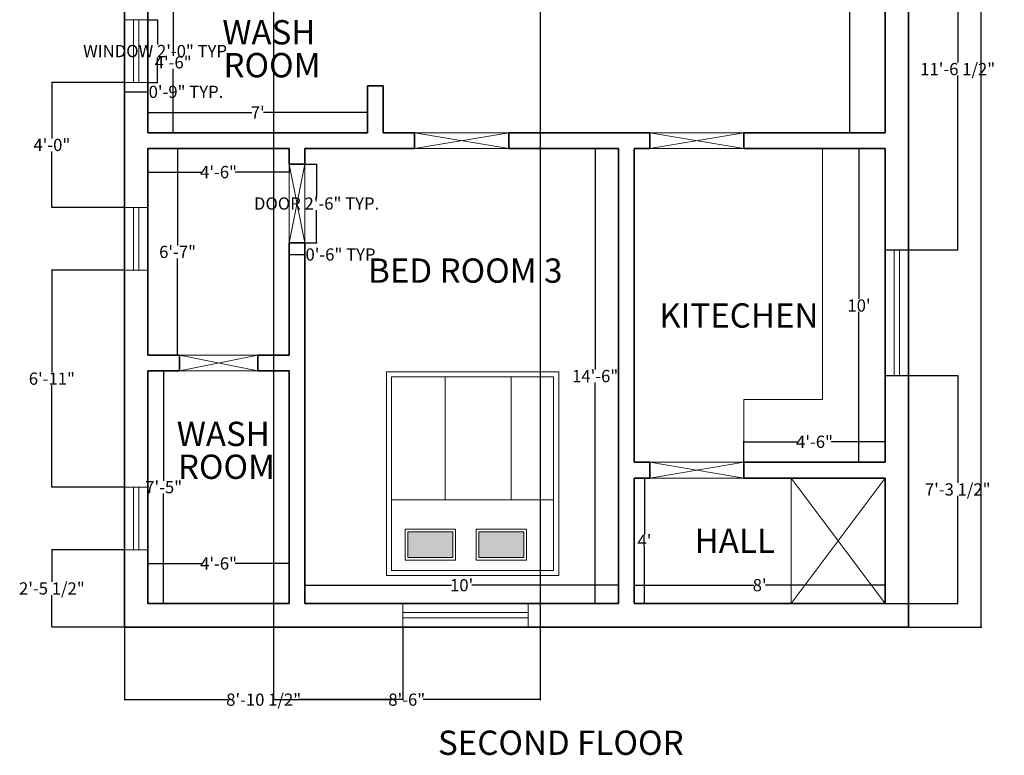
# Model space of a CAD drawing. Units: inches. Extents: x 292 to 2219, y -44 to 516.
# Tile 3 of 4: x 1030 to 1407, y -44 to 237. Entities that reach past the tile are written whole.
import ezdxf

# ---------------------------------------------------------------- set-up
doc = ezdxf.new("R2010")
doc.units = ezdxf.units.IN
doc.header["$MEASUREMENT"] = 0
for name, color, linetype, lineweight in [('A-ANNO-DIMS', 2, 'Continuous', 13), ('A-ANNO-TEXT', 7, 'Continuous', 25), ('A-AREA-IDEN', 7, 'Continuous', 18), ('A-DOOR', 34, 'Continuous', 20), ('A-FLOR-CASE', 9, 'Continuous', 18), ('A-FLOR-OPEN', 7, 'Continuous', 18), ('A-FURN', 8, 'Continuous', 18), ('A-GLAZ', 34, 'Continuous', 18), ('A-WALL', 7, 'Continuous', 35)]:
    doc.layers.add(name, color=color, linetype=linetype, lineweight=lineweight)
doc.styles.get("Standard").update_dxf_attribs({"font": 'arial.ttf'})
doc.dimstyles.get("Standard").update_dxf_attribs({"dimtxt": 4.68, "dimasz": 0.18, "dimexe": 0.18, "dimexo": 0.0625, "dimgap": 0.09, "dimtad": 0, "dimtih": 1, "dimtoh": 1, "dimdec": 0, "dimzin": 0, "dimdsep": 46, "dimlunit": 3, "dimtxsty": 'Standard', "dimcen": 0.09, "dimadec": 0, "dimazin": 0, "dimtfac": 1, "dimtdec": 0, "dimtofl": 0, "dimtmove": 0, "dimatfit": 3, "dimfxl": 1, "dimtolj": 1, "dimtzin": 0, "dimarcsym": 0})

# ---------------------------------------------------------------- blocks, each defined once
blk = doc.blocks.new('*D21')
at = {"layer": 'A-ANNO-DIMS', "color": 0, "lineweight": -2, "transparency": 16777216}
for p, q in [((1079.18, 247.82), (1088.93, 247.82)), ((1088.75, 247.64), (1088.75, 223.3)), ((1088.75, 194), (1088.75, 218.34)), ((1079.18, 193.82), (1088.93, 193.82))]:
    blk.add_line(p, q, dxfattribs=at)
at = {"layer": 'A-ANNO-DIMS', "color": 0, "transparency": 16777216}
for points in [[(1088.72, 247.64), (1088.78, 247.64), (1088.75, 247.82)], [(1088.72, 194), (1088.78, 194), (1088.75, 193.82)]]:
    blk.add_solid(points, dxfattribs=at)
at = {"layer": 'Defpoints', "color": 0, "transparency": 16777216}
for p in [(1079.11, 247.82), (1088.75, 247.82), (1079.11, 193.82)]:
    blk.add_point(p, dxfattribs=at)
at = {"layer": 'A-ANNO-DIMS', "color": 0, "transparency": 16777216, "insert": (1088.75, 220.82), "char_height": 4.68, "attachment_point": 5}
blk.add_mtext('\\A1;4\'-6"', dxfattribs=at)
blk = doc.blocks.new('*D22')
at = {"layer": 'A-ANNO-DIMS', "color": 0, "lineweight": -2, "transparency": 16777216}
for p, q in [((1079.11, 193.88), (1079.11, 201.82)), ((1079.29, 201.64), (1118.89, 201.64)), ((1162.93, 201.64), (1123.34, 201.64)), ((1163.11, 193.88), (1163.11, 201.82))]:
    blk.add_line(p, q, dxfattribs=at)
at = {"layer": 'A-ANNO-DIMS', "color": 0, "transparency": 16777216}
for points in [[(1079.29, 201.67), (1079.29, 201.61), (1079.11, 201.64)], [(1162.93, 201.67), (1162.93, 201.61), (1163.11, 201.64)]]:
    blk.add_solid(points, dxfattribs=at)
at = {"layer": 'Defpoints', "color": 0, "transparency": 16777216}
for p in [(1163.11, 201.64), (1079.11, 193.82), (1163.11, 193.82)]:
    blk.add_point(p, dxfattribs=at)
at = {"layer": 'A-ANNO-DIMS', "color": 0, "transparency": 16777216, "insert": (1121.11, 201.64), "char_height": 4.68, "attachment_point": 5}
blk.add_mtext("\\A1;7'", dxfattribs=at)
blk = doc.blocks.new('*D23')
at = {"layer": 'A-ANNO-DIMS', "color": 0, "lineweight": -2, "transparency": 16777216}
for p, q in [((1079.18, 187.82), (1090.61, 187.82)), ((1090.43, 187.64), (1090.43, 150.8)), ((1090.43, 109), (1090.43, 145.84)), ((1079.18, 108.82), (1090.61, 108.82))]:
    blk.add_line(p, q, dxfattribs=at)
at = {"layer": 'A-ANNO-DIMS', "color": 0, "transparency": 16777216}
for points in [[(1090.4, 187.64), (1090.46, 187.64), (1090.43, 187.82)], [(1090.4, 109), (1090.46, 109), (1090.43, 108.82)]]:
    blk.add_solid(points, dxfattribs=at)
at = {"layer": 'Defpoints', "color": 0, "transparency": 16777216}
for p in [(1079.11, 187.82), (1090.43, 187.82), (1079.11, 108.82)]:
    blk.add_point(p, dxfattribs=at)
at = {"layer": 'A-ANNO-DIMS', "color": 0, "transparency": 16777216, "insert": (1090.43, 148.32), "char_height": 4.68, "attachment_point": 5}
blk.add_mtext('\\A1;6\'-7"', dxfattribs=at)
blk = doc.blocks.new('*D24')
at = {"layer": 'A-ANNO-DIMS', "color": 0, "lineweight": -2, "transparency": 16777216}
for p, q in [((1079.11, 187.75), (1079.11, 178.67)), ((1133.11, 187.75), (1133.11, 178.67)), ((1079.29, 178.85), (1099.71, 178.85)), ((1132.93, 178.85), (1112.52, 178.85))]:
    blk.add_line(p, q, dxfattribs=at)
at = {"layer": 'A-ANNO-DIMS', "color": 0, "transparency": 16777216}
for points in [[(1079.29, 178.88), (1079.29, 178.82), (1079.11, 178.85)], [(1132.93, 178.88), (1132.93, 178.82), (1133.11, 178.85)]]:
    blk.add_solid(points, dxfattribs=at)
at = {"layer": 'Defpoints', "color": 0, "transparency": 16777216}
for p in [(1079.11, 187.82), (1133.11, 187.82), (1133.11, 178.85)]:
    blk.add_point(p, dxfattribs=at)
at = {"layer": 'A-ANNO-DIMS', "color": 0, "transparency": 16777216, "insert": (1106.11, 178.85), "char_height": 4.68, "attachment_point": 5}
blk.add_mtext('\\A1;4\'-6"', dxfattribs=at)
blk = doc.blocks.new('*D25')
at = {"layer": 'A-ANNO-DIMS', "color": 0, "lineweight": -2, "transparency": 16777216}
for p, q in [((1079.11, 13.88), (1079.11, 29.3)), ((1079.29, 29.12), (1099.71, 29.12)), ((1132.93, 29.12), (1112.52, 29.12)), ((1133.11, 13.88), (1133.11, 29.3))]:
    blk.add_line(p, q, dxfattribs=at)
at = {"layer": 'A-ANNO-DIMS', "color": 0, "transparency": 16777216}
for points in [[(1079.29, 29.15), (1079.29, 29.09), (1079.11, 29.12)], [(1132.93, 29.15), (1132.93, 29.09), (1133.11, 29.12)]]:
    blk.add_solid(points, dxfattribs=at)
at = {"layer": 'Defpoints', "color": 0, "transparency": 16777216}
for p in [(1133.11, 29.12), (1079.11, 13.82), (1133.11, 13.82)]:
    blk.add_point(p, dxfattribs=at)
at = {"layer": 'A-ANNO-DIMS', "color": 0, "transparency": 16777216, "insert": (1106.11, 29.12), "char_height": 4.68, "attachment_point": 5}
blk.add_mtext('\\A1;4\'-6"', dxfattribs=at)
blk = doc.blocks.new('*D26')
at = {"layer": 'A-ANNO-DIMS', "color": 0, "lineweight": -2, "transparency": 16777216}
for p, q in [((1079.18, 102.82), (1085.29, 102.82)), ((1085.11, 102.64), (1085.11, 60.79)), ((1085.11, 14), (1085.11, 55.85)), ((1079.18, 13.82), (1085.29, 13.82))]:
    blk.add_line(p, q, dxfattribs=at)
at = {"layer": 'A-ANNO-DIMS', "color": 0, "transparency": 16777216}
for points in [[(1085.08, 102.64), (1085.14, 102.64), (1085.11, 102.82)], [(1085.08, 14), (1085.14, 14), (1085.11, 13.82)]]:
    blk.add_solid(points, dxfattribs=at)
at = {"layer": 'Defpoints', "color": 0, "transparency": 16777216}
for p in [(1079.11, 102.82), (1085.11, 102.82), (1079.11, 13.82)]:
    blk.add_point(p, dxfattribs=at)
at = {"layer": 'A-ANNO-DIMS', "color": 0, "transparency": 16777216, "insert": (1085.11, 58.32), "char_height": 4.68, "attachment_point": 5}
blk.add_mtext('\\A1;7\'-5"', dxfattribs=at)
blk = doc.blocks.new('*D27')
at = {"layer": 'A-ANNO-DIMS', "color": 0, "lineweight": -2, "transparency": 16777216}
for p, q in [((1139.11, 13.88), (1139.11, 21.01)), ((1139.29, 20.83), (1195.27, 20.83)), ((1258.93, 20.83), (1202.95, 20.83)), ((1259.11, 13.88), (1259.11, 21.01))]:
    blk.add_line(p, q, dxfattribs=at)
at = {"layer": 'A-ANNO-DIMS', "color": 0, "transparency": 16777216}
for points in [[(1139.29, 20.86), (1139.29, 20.8), (1139.11, 20.83)], [(1258.93, 20.86), (1258.93, 20.8), (1259.11, 20.83)]]:
    blk.add_solid(points, dxfattribs=at)
at = {"layer": 'Defpoints', "color": 0, "transparency": 16777216}
for p in [(1259.11, 20.83), (1139.11, 13.82), (1259.11, 13.82)]:
    blk.add_point(p, dxfattribs=at)
at = {"layer": 'A-ANNO-DIMS', "color": 0, "transparency": 16777216, "insert": (1199.11, 20.83), "char_height": 4.68, "attachment_point": 5}
blk.add_mtext("\\A1;10'", dxfattribs=at)
blk = doc.blocks.new('*D28')
at = {"layer": 'A-ANNO-DIMS', "color": 0, "lineweight": -2, "transparency": 16777216}
for p, q in [((1259.05, 187.82), (1250.01, 187.82)), ((1250.19, 187.64), (1250.19, 103.3)), ((1250.19, 14), (1250.19, 98.34)), ((1259.05, 13.82), (1250.01, 13.82))]:
    blk.add_line(p, q, dxfattribs=at)
at = {"layer": 'A-ANNO-DIMS', "color": 0, "transparency": 16777216}
for points in [[(1250.16, 187.64), (1250.22, 187.64), (1250.19, 187.82)], [(1250.16, 14), (1250.22, 14), (1250.19, 13.82)]]:
    blk.add_solid(points, dxfattribs=at)
at = {"layer": 'Defpoints', "color": 0, "transparency": 16777216}
for p in [(1250.19, 187.82), (1259.11, 187.82), (1259.11, 13.82)]:
    blk.add_point(p, dxfattribs=at)
at = {"layer": 'A-ANNO-DIMS', "color": 0, "transparency": 16777216, "insert": (1250.19, 100.82), "char_height": 4.68, "attachment_point": 5}
blk.add_mtext('\\A1;14\'-6"', dxfattribs=at)
blk = doc.blocks.new('*D29')
at = {"layer": 'A-ANNO-DIMS', "color": 0, "lineweight": -2, "transparency": 16777216}
for p, q in [((1265.11, 13.88), (1265.11, 21.01)), ((1265.29, 20.83), (1310.87, 20.83)), ((1360.93, 20.83), (1315.36, 20.83)), ((1361.11, 13.88), (1361.11, 21.01))]:
    blk.add_line(p, q, dxfattribs=at)
at = {"layer": 'A-ANNO-DIMS', "color": 0, "transparency": 16777216}
for points in [[(1265.29, 20.86), (1265.29, 20.8), (1265.11, 20.83)], [(1360.93, 20.86), (1360.93, 20.8), (1361.11, 20.83)]]:
    blk.add_solid(points, dxfattribs=at)
at = {"layer": 'Defpoints', "color": 0, "transparency": 16777216}
for p in [(1361.11, 20.83), (1265.11, 13.82), (1361.11, 13.82)]:
    blk.add_point(p, dxfattribs=at)
at = {"layer": 'A-ANNO-DIMS', "color": 0, "transparency": 16777216, "insert": (1313.11, 20.83), "char_height": 4.68, "attachment_point": 5}
blk.add_mtext("\\A1;8'", dxfattribs=at)
blk = doc.blocks.new('*D30')
at = {"layer": 'A-ANNO-DIMS', "color": 0, "lineweight": -2, "transparency": 16777216}
for p, q in [((1265.18, 61.82), (1269.22, 61.82)), ((1269.04, 61.64), (1269.04, 40.25)), ((1269.04, 14), (1269.04, 35.39)), ((1265.18, 13.82), (1269.22, 13.82))]:
    blk.add_line(p, q, dxfattribs=at)
at = {"layer": 'A-ANNO-DIMS', "color": 0, "transparency": 16777216}
for points in [[(1269.01, 61.64), (1269.07, 61.64), (1269.04, 61.82)], [(1269.01, 14), (1269.07, 14), (1269.04, 13.82)]]:
    blk.add_solid(points, dxfattribs=at)
at = {"layer": 'Defpoints', "color": 0, "transparency": 16777216}
for p in [(1265.11, 61.82), (1269.04, 61.82), (1265.11, 13.82)]:
    blk.add_point(p, dxfattribs=at)
at = {"layer": 'A-ANNO-DIMS', "color": 0, "transparency": 16777216, "insert": (1269.04, 37.82), "char_height": 4.68, "attachment_point": 5}
blk.add_mtext("\\A1;4'", dxfattribs=at)
blk = doc.blocks.new('*D31')
at = {"layer": 'A-ANNO-DIMS', "color": 0, "lineweight": -2, "transparency": 16777216}
for p, q in [((1361.05, 187.82), (1350.94, 187.82)), ((1351.12, 187.64), (1351.12, 130.3)), ((1351.12, 68), (1351.12, 125.34)), ((1361.05, 67.82), (1350.94, 67.82))]:
    blk.add_line(p, q, dxfattribs=at)
at = {"layer": 'A-ANNO-DIMS', "color": 0, "transparency": 16777216}
for points in [[(1351.09, 187.64), (1351.15, 187.64), (1351.12, 187.82)], [(1351.09, 68), (1351.15, 68), (1351.12, 67.82)]]:
    blk.add_solid(points, dxfattribs=at)
at = {"layer": 'Defpoints', "color": 0, "transparency": 16777216}
for p in [(1361.11, 187.82), (1351.12, 67.82), (1361.11, 67.82)]:
    blk.add_point(p, dxfattribs=at)
at = {"layer": 'A-ANNO-DIMS', "color": 0, "transparency": 16777216, "insert": (1351.12, 127.82), "char_height": 4.68, "attachment_point": 5}
blk.add_mtext("\\A1;10'", dxfattribs=at)
blk = doc.blocks.new('*D32')
at = {"layer": 'A-ANNO-DIMS', "color": 0, "lineweight": -2, "transparency": 16777216}
for p, q in [((1307.11, 67.88), (1307.11, 75.86)), ((1307.29, 75.68), (1327.71, 75.68)), ((1360.93, 75.68), (1340.52, 75.68)), ((1361.11, 67.88), (1361.11, 75.86))]:
    blk.add_line(p, q, dxfattribs=at)
at = {"layer": 'A-ANNO-DIMS', "color": 0, "transparency": 16777216}
for points in [[(1307.29, 75.71), (1307.29, 75.65), (1307.11, 75.68)], [(1360.93, 75.71), (1360.93, 75.65), (1361.11, 75.68)]]:
    blk.add_solid(points, dxfattribs=at)
at = {"layer": 'Defpoints', "color": 0, "transparency": 16777216}
for p in [(1361.11, 75.68), (1307.11, 67.82), (1361.11, 67.82)]:
    blk.add_point(p, dxfattribs=at)
at = {"layer": 'A-ANNO-DIMS', "color": 0, "transparency": 16777216, "insert": (1334.11, 75.68), "char_height": 4.68, "attachment_point": 5}
blk.add_mtext('\\A1;4\'-6"', dxfattribs=at)
blk = doc.blocks.new('*D34')
at = {"layer": 'A-ANNO-DIMS', "color": 0, "lineweight": -2, "transparency": 16777216}
for p, q in [((1361.05, 370.82), (1347.49, 370.82)), ((1347.67, 370.64), (1347.67, 284.8)), ((1347.67, 194), (1347.67, 279.84)), ((1361.05, 193.82), (1347.49, 193.82))]:
    blk.add_line(p, q, dxfattribs=at)
at = {"layer": 'A-ANNO-DIMS', "color": 0, "transparency": 16777216}
for points in [[(1347.64, 370.64), (1347.7, 370.64), (1347.67, 370.82)], [(1347.64, 194), (1347.7, 194), (1347.67, 193.82)]]:
    blk.add_solid(points, dxfattribs=at)
at = {"layer": 'Defpoints', "color": 0, "transparency": 16777216}
for p in [(1347.67, 370.82), (1361.11, 370.82), (1361.11, 193.82)]:
    blk.add_point(p, dxfattribs=at)
at = {"layer": 'A-ANNO-DIMS', "color": 0, "transparency": 16777216, "insert": (1347.67, 282.32), "char_height": 4.68, "attachment_point": 5}
blk.add_mtext('\\A1;14\'-9"', dxfattribs=at)
blk = doc.blocks.new('BED-DOUBLE')
h = blk.add_hatch(color=256)
h.dxf.hatch_style = 1
h.paths.add_polyline_path([(6.9, 40.51), (16.75, 40.51), (16.75, 57.79), (6.9, 57.79)])
h.paths.add_polyline_path([(16.75, 30.67), (6.9, 30.67), (6.9, 13.4), (16.75, 13.4)])
for p, q in [((0, 0), (0, 66)), ((0, 66), (78, 66)), ((78, 66), (78, 0)), ((2, 64), (76, 64)), ((2, 2), (2, 64)), ((29, 2), (29, 64)), ((76, 64), (76, 2)), ((76, 43.53), (29, 43.53)), ((76, 18.22), (29, 18.22)), ((78, 0), (0, 0)), ((76, 2), (2, 2))]:
    blk.add_line(p, q)
for points in [[(5.9, 58.79), (17.75, 58.79), (17.75, 39.51), (5.9, 39.51)], [(6.9, 57.79), (16.75, 57.79), (16.75, 40.51), (6.9, 40.51)], [(5.9, 31.67), (17.75, 31.67), (17.75, 12.4), (5.9, 12.4)], [(6.9, 30.67), (16.75, 30.67), (16.75, 13.4), (6.9, 13.4)]]:
    blk.add_lwpolyline(points, close=True)
blk = doc.blocks.new('WIN-48')
for p, q in [((0, 48), (9, 48)), ((0, 0), (0, 48)), ((3.5, 48), (3.5, 0)), ((5.5, 48), (5.5, 0)), ((9, 48), (9, 0)), ((9, 0), (0, 0))]:
    blk.add_line(p, q)
blk = doc.blocks.new('DOOR-36')
for p, q in [((0, 36), (6, 36)), ((0, 0), (6, 36)), ((6, 0), (0, 36)), ((0, 36), (0, 0)), ((6, 36), (6, 0)), ((0, 0), (6, 0))]:
    blk.add_line(p, q)
blk = doc.blocks.new('WIN-24')
for p, q in [((0, 24), (9, 24)), ((0, 24), (0, 0)), ((3.5, 24), (3.5, 0)), ((5.5, 24), (5.5, 0)), ((9, 24), (9, 0)), ((0, 0), (9, 0))]:
    blk.add_line(p, q)
blk = doc.blocks.new('DOOR-30')
for p, q in [((0, 30), (6, 30)), ((0, 30), (6, 0)), ((6, 30), (0, 0)), ((0, 0), (0, 30)), ((6, 0), (6, 30)), ((0, 0), (6, 0))]:
    blk.add_line(p, q)
blk = doc.blocks.new('FLOOR-OPENING-36X48')
for p, q in [((0, 48), (0, 0)), ((0, 48), (36, 0)), ((36, 48), (0, 0))]:
    blk.add_line(p, q)
blk = doc.blocks.new('*D46')
at = {"layer": 'A-ANNO-DIMS', "color": 0, "lineweight": -2, "transparency": 16777216}
for p, q in [((1079.18, 237.14), (1082.89, 237.14)), ((1082.71, 236.96), (1082.71, 227.65)), ((1082.71, 213.32), (1082.71, 222.62)), ((1079.18, 213.14), (1082.89, 213.14))]:
    blk.add_line(p, q, dxfattribs=at)
at = {"layer": 'A-ANNO-DIMS', "color": 0, "transparency": 16777216}
for points in [[(1082.68, 236.96), (1082.74, 236.96), (1082.71, 237.14)], [(1082.68, 213.32), (1082.74, 213.32), (1082.71, 213.14)]]:
    blk.add_solid(points, dxfattribs=at)
at = {"layer": 'Defpoints', "color": 0, "transparency": 16777216}
for p in [(1079.11, 237.14), (1082.71, 237.14), (1079.11, 213.14)]:
    blk.add_point(p, dxfattribs=at)
at = {"layer": 'A-ANNO-DIMS', "color": 0, "transparency": 16777216, "insert": (1082.71, 225.14), "char_height": 4.68, "attachment_point": 5}
blk.add_mtext('\\A1;WINDOW 2\'-0" TYP.', dxfattribs=at)
blk = doc.blocks.new('*D47')
at = {"layer": 'A-ANNO-DIMS', "color": 0, "lineweight": -2, "transparency": 16777216}
for p, q in [((1070.11, 213.07), (1070.11, 209.36)), ((1079.11, 213.07), (1079.11, 209.36)), ((1070.29, 209.54), (1078.93, 209.54)), ((1079.11, 209.54), (1079.29, 209.54))]:
    blk.add_line(p, q, dxfattribs=at)
at = {"layer": 'A-ANNO-DIMS', "color": 0, "transparency": 16777216}
for points in [[(1070.29, 209.57), (1070.29, 209.51), (1070.11, 209.54)], [(1078.93, 209.57), (1078.93, 209.51), (1079.11, 209.54)]]:
    blk.add_solid(points, dxfattribs=at)
at = {"layer": 'Defpoints', "color": 0, "transparency": 16777216}
for p in [(1070.11, 213.14), (1079.11, 213.14), (1079.11, 209.54)]:
    blk.add_point(p, dxfattribs=at)
at = {"layer": 'A-ANNO-DIMS', "color": 0, "transparency": 16777216, "insert": (1093.65, 209.54), "char_height": 4.68, "attachment_point": 5}
blk.add_mtext('\\A1;0\'-9" TYP.', dxfattribs=at)
blk = doc.blocks.new('*D50')
at = {"layer": 'A-ANNO-DIMS', "color": 0, "lineweight": -2, "transparency": 16777216}
for p, q in [((1139.18, 181.82), (1143.79, 181.82)), ((1143.61, 181.64), (1143.61, 169.33)), ((1143.61, 152), (1143.61, 164.3)), ((1139.18, 151.82), (1143.79, 151.82))]:
    blk.add_line(p, q, dxfattribs=at)
at = {"layer": 'A-ANNO-DIMS', "color": 0, "transparency": 16777216}
for points in [[(1143.58, 181.64), (1143.64, 181.64), (1143.61, 181.82)], [(1143.58, 152), (1143.64, 152), (1143.61, 151.82)]]:
    blk.add_solid(points, dxfattribs=at)
at = {"layer": 'Defpoints', "color": 0, "transparency": 16777216}
for p in [(1139.11, 181.82), (1143.61, 181.82), (1139.11, 151.82)]:
    blk.add_point(p, dxfattribs=at)
at = {"layer": 'A-ANNO-DIMS', "color": 0, "transparency": 16777216, "insert": (1143.61, 166.82), "char_height": 4.68, "attachment_point": 5}
blk.add_mtext('\\A1;DOOR 2\'-6" TYP.', dxfattribs=at)
blk = doc.blocks.new('*D51')
at = {"layer": 'A-ANNO-DIMS', "color": 0, "lineweight": -2, "transparency": 16777216}
for p, q in [((1133.11, 151.75), (1133.11, 147.14)), ((1139.11, 151.75), (1139.11, 147.14)), ((1133.29, 147.32), (1138.93, 147.32)), ((1139.11, 147.32), (1139.29, 147.32))]:
    blk.add_line(p, q, dxfattribs=at)
at = {"layer": 'A-ANNO-DIMS', "color": 0, "transparency": 16777216}
for points in [[(1133.29, 147.35), (1133.29, 147.29), (1133.11, 147.32)], [(1138.93, 147.35), (1138.93, 147.29), (1139.11, 147.32)]]:
    blk.add_solid(points, dxfattribs=at)
at = {"layer": 'Defpoints', "color": 0, "transparency": 16777216}
for p in [(1133.11, 151.82), (1139.11, 151.82), (1139.11, 147.32)]:
    blk.add_point(p, dxfattribs=at)
at = {"layer": 'A-ANNO-DIMS', "color": 0, "transparency": 16777216, "insert": (1153.65, 147.32), "char_height": 4.68, "attachment_point": 5}
blk.add_mtext('\\A1;0\'-6" TYP.', dxfattribs=at)
blk = doc.blocks.new('*D65')
at = {"layer": 'A-ANNO-DIMS', "color": 0, "lineweight": -2, "transparency": 16777216}
for p, q in [((1070.11, 4.75), (1070.11, -23.14)), ((1176.62, 4.75), (1176.62, -23.14)), ((1070.29, -22.96), (1109.78, -22.96)), ((1176.44, -22.96), (1136.95, -22.96))]:
    blk.add_line(p, q, dxfattribs=at)
at = {"layer": 'A-ANNO-DIMS', "color": 0, "transparency": 16777216}
for points in [[(1070.29, -22.93), (1070.29, -22.99), (1070.11, -22.96)], [(1176.44, -22.93), (1176.44, -22.99), (1176.62, -22.96)]]:
    blk.add_solid(points, dxfattribs=at)
at = {"layer": 'Defpoints', "color": 0, "transparency": 16777216}
for p in [(1070.11, 4.82), (1176.62, 4.82), (1176.62, -22.96)]:
    blk.add_point(p, dxfattribs=at)
at = {"layer": 'A-ANNO-DIMS', "color": 0, "transparency": 16777216, "insert": (1123.37, -22.96), "char_height": 4.68, "attachment_point": 5}
blk.add_mtext('\\A1;8\'-10 1/2"', dxfattribs=at)
blk = doc.blocks.new('*D66')
at = {"layer": 'A-ANNO-DIMS', "color": 0, "lineweight": -2, "transparency": 16777216}
for p, q in [((1070.05, 34.32), (1042.16, 34.32)), ((1042.34, 34.14), (1042.34, 22.08)), ((1042.34, 5), (1042.34, 17.06)), ((1070.05, 4.82), (1042.16, 4.82))]:
    blk.add_line(p, q, dxfattribs=at)
at = {"layer": 'A-ANNO-DIMS', "color": 0, "transparency": 16777216}
for points in [[(1042.31, 34.14), (1042.37, 34.14), (1042.34, 34.32)], [(1042.31, 5), (1042.37, 5), (1042.34, 4.82)]]:
    blk.add_solid(points, dxfattribs=at)
at = {"layer": 'Defpoints', "color": 0, "transparency": 16777216}
for p in [(1042.34, 34.32), (1070.11, 34.32), (1070.11, 4.82)]:
    blk.add_point(p, dxfattribs=at)
at = {"layer": 'A-ANNO-DIMS', "color": 0, "transparency": 16777216, "insert": (1042.34, 19.57), "char_height": 4.68, "attachment_point": 5}
blk.add_mtext('\\A1;2\'-5 1/2"', dxfattribs=at)
blk = doc.blocks.new('*D67')
at = {"layer": 'A-ANNO-DIMS', "color": 0, "lineweight": -2, "transparency": 16777216}
for p, q in [((1070.05, 141.35), (1042.16, 141.35)), ((1042.34, 141.17), (1042.34, 102.31)), ((1042.34, 58.5), (1042.34, 97.35)), ((1070.05, 58.32), (1042.16, 58.32))]:
    blk.add_line(p, q, dxfattribs=at)
at = {"layer": 'A-ANNO-DIMS', "color": 0, "transparency": 16777216}
for points in [[(1042.31, 141.17), (1042.37, 141.17), (1042.34, 141.35)], [(1042.31, 58.5), (1042.37, 58.5), (1042.34, 58.32)]]:
    blk.add_solid(points, dxfattribs=at)
at = {"layer": 'Defpoints', "color": 0, "transparency": 16777216}
for p in [(1042.34, 141.35), (1070.11, 141.35), (1070.11, 58.32)]:
    blk.add_point(p, dxfattribs=at)
at = {"layer": 'A-ANNO-DIMS', "color": 0, "transparency": 16777216, "insert": (1042.34, 99.83), "char_height": 4.68, "attachment_point": 5}
blk.add_mtext('\\A1;6\'-11"', dxfattribs=at)
blk = doc.blocks.new('*D68')
at = {"layer": 'A-ANNO-DIMS', "color": 0, "lineweight": -2, "transparency": 16777216}
for p, q in [((1070.05, 213.14), (1042.16, 213.14)), ((1042.34, 212.96), (1042.34, 191.72)), ((1042.34, 165.53), (1042.34, 186.76)), ((1070.05, 165.35), (1042.16, 165.35))]:
    blk.add_line(p, q, dxfattribs=at)
at = {"layer": 'A-ANNO-DIMS', "color": 0, "transparency": 16777216}
for points in [[(1042.31, 212.96), (1042.37, 212.96), (1042.34, 213.14)], [(1042.31, 165.53), (1042.37, 165.53), (1042.34, 165.35)]]:
    blk.add_solid(points, dxfattribs=at)
at = {"layer": 'Defpoints', "color": 0, "transparency": 16777216}
for p in [(1042.34, 213.14), (1070.11, 213.14), (1070.11, 165.35)]:
    blk.add_point(p, dxfattribs=at)
at = {"layer": 'A-ANNO-DIMS', "color": 0, "transparency": 16777216, "insert": (1042.34, 189.24), "char_height": 4.68, "attachment_point": 5}
blk.add_mtext('\\A1;4\'-0"', dxfattribs=at)
blk = doc.blocks.new('*D70')
at = {"layer": 'A-ANNO-DIMS', "color": 0, "lineweight": -2, "transparency": 16777216}
for p, q in [((1361.18, 101.08), (1389.07, 101.08)), ((1388.89, 100.9), (1388.89, 59.96)), ((1388.89, 14), (1388.89, 54.94)), ((1361.18, 13.82), (1389.07, 13.82))]:
    blk.add_line(p, q, dxfattribs=at)
at = {"layer": 'A-ANNO-DIMS', "color": 0, "transparency": 16777216}
for points in [[(1388.86, 100.9), (1388.92, 100.9), (1388.89, 101.08)], [(1388.86, 14), (1388.92, 14), (1388.89, 13.82)]]:
    blk.add_solid(points, dxfattribs=at)
at = {"layer": 'Defpoints', "color": 0, "transparency": 16777216}
for p in [(1361.11, 101.08), (1361.11, 13.82), (1388.89, 13.82)]:
    blk.add_point(p, dxfattribs=at)
at = {"layer": 'A-ANNO-DIMS', "color": 0, "transparency": 16777216, "insert": (1388.89, 57.45), "char_height": 4.68, "attachment_point": 5}
blk.add_mtext('\\A1;7\'-3 1/2"', dxfattribs=at)
blk = doc.blocks.new('*D71')
at = {"layer": 'A-ANNO-DIMS', "color": 0, "lineweight": -2, "transparency": 16777216}
for p, q in [((1361.18, 287.41), (1389.07, 287.41)), ((1388.89, 287.23), (1388.89, 220.75)), ((1388.89, 149.26), (1388.89, 215.73)), ((1361.18, 149.08), (1389.07, 149.08))]:
    blk.add_line(p, q, dxfattribs=at)
at = {"layer": 'A-ANNO-DIMS', "color": 0, "transparency": 16777216}
for points in [[(1388.86, 287.23), (1388.92, 287.23), (1388.89, 287.41)], [(1388.86, 149.26), (1388.92, 149.26), (1388.89, 149.08)]]:
    blk.add_solid(points, dxfattribs=at)
at = {"layer": 'Defpoints', "color": 0, "transparency": 16777216}
for p in [(1361.11, 287.41), (1361.11, 149.08), (1388.89, 149.08)]:
    blk.add_point(p, dxfattribs=at)
at = {"layer": 'A-ANNO-DIMS', "color": 0, "transparency": 16777216, "insert": (1388.89, 218.24), "char_height": 4.68, "attachment_point": 5}
blk.add_mtext('\\A1;11\'-6 1/2"', dxfattribs=at)
blk = doc.blocks.new('*D73')
at = {"layer": 'A-ANNO-DIMS', "color": 0, "lineweight": -2, "transparency": 16777216}
for p, q in [((1127.11, 475.75), (1127.11, -23.14)), ((1229.11, 475.75), (1229.11, -23.14)), ((1127.29, -22.96), (1171.8, -22.96)), ((1228.93, -22.96), (1184.43, -22.96))]:
    blk.add_line(p, q, dxfattribs=at)
at = {"layer": 'A-ANNO-DIMS', "color": 0, "transparency": 16777216}
for points in [[(1127.29, -22.93), (1127.29, -22.99), (1127.11, -22.96)], [(1228.93, -22.93), (1228.93, -22.99), (1229.11, -22.96)]]:
    blk.add_solid(points, dxfattribs=at)
at = {"layer": 'Defpoints', "color": 0, "transparency": 16777216}
for p in [(1127.11, 475.82), (1229.11, 475.82), (1229.11, -22.96)]:
    blk.add_point(p, dxfattribs=at)
at = {"layer": 'A-ANNO-DIMS', "color": 0, "transparency": 16777216, "insert": (1178.11, -22.96), "char_height": 4.68, "attachment_point": 5}
blk.add_mtext('\\A1;8\'-6"', dxfattribs=at)
blk = doc.blocks.new('*D75')
at = {"layer": 'A-ANNO-DIMS', "color": 0, "lineweight": -2, "transparency": 16777216}
for p, q in [((1370.18, 484.82), (1398.07, 484.82)), ((1397.89, 484.64), (1397.89, 247.3)), ((1397.89, 5), (1397.89, 242.34)), ((1370.18, 4.82), (1398.07, 4.82))]:
    blk.add_line(p, q, dxfattribs=at)
at = {"layer": 'A-ANNO-DIMS', "color": 0, "transparency": 16777216}
for points in [[(1397.86, 484.64), (1397.92, 484.64), (1397.89, 484.82)], [(1397.86, 5), (1397.92, 5), (1397.89, 4.82)]]:
    blk.add_solid(points, dxfattribs=at)
at = {"layer": 'Defpoints', "color": 0, "transparency": 16777216}
for p in [(1370.11, 484.82), (1397.89, 484.82), (1370.11, 4.82)]:
    blk.add_point(p, dxfattribs=at)
at = {"layer": 'A-ANNO-DIMS', "color": 0, "transparency": 16777216, "insert": (1397.89, 244.82), "char_height": 4.68, "attachment_point": 5}
blk.add_mtext('\\A1;40\'-0"', dxfattribs=at)

msp = doc.modelspace()

# ---------------------------------------------------------------- linework, layer by layer
at = {"layer": 'A-FLOR-CASE'}
for p, q in [((1337.11, 187.82), (1337.11, 91.82)), ((1307.11, 91.82), (1337.11, 91.82)), ((1307.11, 91.82), (1307.11, 67.82))]:
    msp.add_line(p, q, dxfattribs=at)
at = {"layer": 'A-WALL'}
for p, q in [((1070.11, 4.82), (1070.11, 484.82)), ((1370.11, 484.82), (1370.11, 4.82)), ((1361.11, 370.82), (1361.11, 193.82)), ((1079.11, 193.82), (1079.11, 247.82)), ((1079.11, 199.82), (1079.11, 247.82)), ((1163.11, 193.82), (1163.11, 211.82)), ((1163.11, 211.82), (1169.11, 211.82)), ((1169.11, 193.82), (1169.11, 211.82)), ((1079.11, 193.82), (1163.11, 193.82)), ((1169.11, 193.82), (1181.11, 193.82)), ((1181.11, 193.82), (1181.11, 187.82)), ((1217.11, 193.82), (1217.11, 187.82)), ((1217.11, 193.82), (1271.11, 193.82)), ((1271.11, 187.82), (1271.11, 193.82)), ((1307.11, 193.82), (1361.11, 193.82)), ((1307.11, 187.82), (1307.11, 193.82)), ((1079.11, 108.82), (1079.11, 187.82)), ((1079.11, 108.82), (1079.11, 187.82)), ((1079.11, 187.82), (1133.11, 187.82)), ((1133.11, 181.82), (1133.11, 187.82)), ((1139.11, 181.82), (1139.11, 187.82)), ((1139.11, 187.82), (1181.11, 187.82)), ((1217.11, 187.82), (1259.11, 187.82)), ((1259.11, 13.82), (1259.11, 187.82)), ((1265.11, 187.82), (1271.11, 187.82)), ((1265.11, 67.82), (1265.11, 187.82)), ((1307.11, 187.82), (1361.11, 187.82)), ((1361.11, 187.82), (1361.11, 67.82)), ((1133.11, 181.82), (1139.11, 181.82)), ((1133.11, 108.82), (1133.11, 151.82)), ((1133.11, 151.82), (1139.11, 151.82)), ((1139.11, 13.82), (1139.11, 151.82)), ((1079.11, 108.82), (1091.11, 108.82)), ((1091.11, 102.82), (1091.11, 108.82)), ((1121.11, 102.82), (1121.11, 108.82)), ((1121.11, 108.82), (1133.11, 108.82)), ((1079.11, 13.82), (1079.11, 102.82)), ((1079.11, 13.82), (1079.11, 102.82)), ((1079.11, 102.82), (1091.11, 102.82)), ((1121.11, 102.82), (1133.11, 102.82)), ((1133.11, 13.82), (1133.11, 102.82)), ((1265.11, 67.82), (1271.11, 67.82)), ((1271.11, 61.82), (1271.11, 67.82)), ((1307.11, 61.82), (1307.11, 67.82)), ((1307.11, 67.82), (1361.11, 67.82)), ((1265.11, 13.82), (1265.11, 61.82)), ((1265.11, 61.82), (1271.11, 61.82)), ((1307.11, 61.82), (1361.11, 61.82)), ((1361.11, 61.82), (1361.11, 13.82)), ((1079.11, 13.82), (1133.11, 13.82)), ((1139.11, 13.82), (1259.11, 13.82)), ((1265.11, 13.82), (1361.11, 13.82)), ((1070.11, 4.82), (1370.11, 4.82))]:
    msp.add_line(p, q, dxfattribs=at)

# ---------------------------------------------------------------- block references
at = {"layer": 'A-DOOR'}
for name, p, rotation in [('DOOR-36', (1217.11, 187.82), 90.00000000000033), ('DOOR-36', (1307.11, 187.82), 90.00000000000055), ('DOOR-30', (1091.11, 108.82), 270.0000000000009), ('DOOR-36', (1307.11, 61.82), 90.00000000000048)]:
    msp.add_blockref(name, p, dxfattribs=dict(at, rotation=rotation))
msp.add_blockref('DOOR-30', (1133.11, 151.82), dxfattribs=at)
at = {"layer": 'A-FLOR-OPEN'}
msp.add_blockref('FLOOR-OPENING-36X48', (1325.11, 13.82), dxfattribs=at)
at = {"layer": 'A-FURN', "rotation": 90.00000000000018}
msp.add_blockref('BED-DOUBLE', (1236.31, 24.48), dxfattribs=at)
at = {"layer": 'A-GLAZ'}
for name, p in [('WIN-24', (1070.11, 213.13)), ('WIN-24', (1070.11, 141.35)), ('WIN-48', (1361.11, 101.08)), ('WIN-24', (1070.11, 34.32))]:
    msp.add_blockref(name, p, dxfattribs=at)
at = {"layer": 'A-GLAZ', "rotation": 270}
msp.add_blockref('WIN-48', (1176.62, 13.82), dxfattribs=at)

# ---------------------------------------------------------------- texts
at = {"layer": 'A-ANNO-TEXT'}
msp.add_text('SECOND FLOOR ', height=9.289, dxfattribs=at).set_placement((1190.07, -44.08))
at = {"layer": 'A-AREA-IDEN'}
for s, p in [('WASH ', (1107.57, 227.68)), ('ROOM', (1107.99, 215.1)), ('BED ROOM 3', (1163.31, 136.52)), ('KITECHEN', (1274.71, 119.35)), ('WASH ', (1090.13, 74.06)), ('ROOM', (1090.55, 61.48)), ('HALL', (1288.26, 33.2))]:
    msp.add_text(s, height=9.289, dxfattribs=at).set_placement(p)

# ---------------------------------------------------------------- dimensions: what is measured, and where the dimension line sits
at = {"layer": 'A-ANNO-DIMS'}
for base, p1, p2, angle, override, picture, middle in [((1397.89, 484.82), (1370.11, 4.82), (1370.11, 484.82), 90, {"dimdec": 1, "dimlfac": 1, "dimrnd": 0, "dimzin": 1, "dimdsep": 46, "dimlunit": 4, "dimfrac": 2}, '*D75', (1397.89, 244.82)), ((1347.67, 370.82), (1361.11, 193.82), (1361.11, 370.82), 90, {"dimclrd": 0, "dimclre": 0, "dimclrt": 0}, '*D34', (1347.67, 282.32)), ((1388.89, 149.08), (1361.11, 287.41), (1361.11, 149.08), 270, {"dimdec": 1, "dimlfac": 1, "dimrnd": 0, "dimzin": 1, "dimdsep": 46, "dimlunit": 4, "dimfrac": 2}, '*D71', (1388.89, 218.24)), ((1088.75, 247.82), (1079.11, 193.82), (1079.11, 247.82), 90, {"dimclrd": 0, "dimclre": 0, "dimclrt": 0}, '*D21', (1088.75, 220.82)), ((1042.34, 213.14), (1070.11, 165.35), (1070.11, 213.14), 90, {"dimdec": 1, "dimlfac": 1, "dimrnd": 0, "dimzin": 1, "dimdsep": 46, "dimlunit": 4, "dimfrac": 2}, '*D68', (1042.34, 189.24)), ((1090.43, 187.82), (1079.11, 108.82), (1079.11, 187.82), 90, {"dimclrd": 0, "dimclre": 0, "dimclrt": 0}, '*D23', (1090.43, 148.32)), ((1250.19, 187.82), (1259.11, 13.82), (1259.11, 187.82), 90, {"dimclrd": 0, "dimclre": 0, "dimclrt": 0}, '*D28', (1250.19, 100.82)), ((1351.12, 67.82), (1361.11, 187.82), (1361.11, 67.82), 90, {"dimclrd": 0, "dimclre": 0, "dimclrt": 0}, '*D31', (1351.12, 127.82)), ((1042.34, 141.35), (1070.11, 58.32), (1070.11, 141.35), 90, {"dimdec": 1, "dimlfac": 1, "dimrnd": 0, "dimzin": 1, "dimdsep": 46, "dimlunit": 4, "dimfrac": 2}, '*D67', (1042.34, 99.83)), ((1085.11, 102.82), (1079.11, 13.82), (1079.11, 102.82), 90, {"dimclrd": 0, "dimclre": 0, "dimclrt": 0}, '*D26', (1085.11, 58.32)), ((1388.89, 13.82), (1361.11, 101.08), (1361.11, 13.82), 270, {"dimdec": 1, "dimlfac": 1, "dimrnd": 0, "dimzin": 1, "dimdsep": 46, "dimlunit": 4, "dimfrac": 2}, '*D70', (1388.89, 57.45)), ((1269.04, 61.82), (1265.11, 13.82), (1265.11, 61.82), 90, {"dimclrd": 0, "dimclre": 0, "dimclrt": 0}, '*D30', (1269.04, 37.82)), ((1042.34, 34.32), (1070.11, 4.82), (1070.11, 34.32), 90, {"dimdec": 1, "dimlfac": 1, "dimrnd": 0, "dimzin": 1, "dimdsep": 46, "dimlunit": 4, "dimfrac": 2}, '*D66', (1042.34, 19.57))]:
    dim = msp.add_linear_dim(base=base, p1=p1, p2=p2, angle=angle, dimstyle='Standard', override=override, dxfattribs=at)
    dim.commit()
    dim.dimension.update_dxf_attribs({"geometry": picture, "text_midpoint": middle})
for base, p1, p2, override, picture, middle in [((1229.11, -22.96), (1127.11, 475.82), (1229.11, 475.82), {"dimdec": 1, "dimlfac": 1, "dimrnd": 0, "dimzin": 1, "dimdsep": 46, "dimlunit": 4, "dimfrac": 2}, '*D73', (1178.11, -22.96)), ((1163.11, 201.64), (1079.11, 193.82), (1163.11, 193.82), {"dimclrd": 0, "dimclre": 0, "dimclrt": 0}, '*D22', (1121.11, 201.64)), ((1133.11, 178.85), (1079.11, 187.82), (1133.11, 187.82), {"dimclrd": 0, "dimclre": 0, "dimclrt": 0}, '*D24', (1106.11, 178.85)), ((1361.11, 75.68), (1307.11, 67.82), (1361.11, 67.82), {"dimclrd": 0, "dimclre": 0, "dimclrt": 0}, '*D32', (1334.11, 75.68)), ((1133.11, 29.12), (1079.11, 13.82), (1133.11, 13.82), {"dimclrd": 0, "dimclre": 0, "dimclrt": 0}, '*D25', (1106.11, 29.12)), ((1259.11, 20.83), (1139.11, 13.82), (1259.11, 13.82), {"dimclrd": 0, "dimclre": 0, "dimclrt": 0}, '*D27', (1199.11, 20.83)), ((1361.11, 20.83), (1265.11, 13.82), (1361.11, 13.82), {"dimclrd": 0, "dimclre": 0, "dimclrt": 0}, '*D29', (1313.11, 20.83)), ((1176.62, -22.96), (1070.11, 4.82), (1176.62, 4.82), {"dimdec": 1, "dimlfac": 1, "dimrnd": 0, "dimzin": 1, "dimdsep": 46, "dimlunit": 4, "dimfrac": 2}, '*D65', (1123.37, -22.96))]:
    dim = msp.add_linear_dim(base=base, p1=p1, p2=p2, dimstyle='Standard', override=override, dxfattribs=at)
    dim.commit()
    dim.dimension.update_dxf_attribs({"geometry": picture, "text_midpoint": middle})
for base, p1, p2, text, picture, middle in [((1082.71, 237.14), (1079.11, 213.14), (1079.11, 237.14), 'WINDOW <> TYP.', '*D46', (1082.71, 225.14)), ((1143.61, 181.82), (1139.11, 151.82), (1139.11, 181.82), 'DOOR <> TYP.', '*D50', (1143.61, 166.82))]:
    dim = msp.add_linear_dim(base=base, p1=p1, p2=p2, angle=90, text=text, dimstyle='Standard', override={"dimdec": 1, "dimlfac": 1, "dimrnd": 0, "dimzin": 1, "dimdsep": 46, "dimlunit": 4, "dimfrac": 2}, dxfattribs=at)
    dim.commit()
    dim.dimension.update_dxf_attribs({"geometry": picture, "text_midpoint": middle})
for base, p1, p2, picture, middle in [((1079.11, 209.54), (1070.11, 213.14), (1079.11, 213.14), '*D47', (1093.65, 209.54)), ((1139.11, 147.32), (1133.11, 151.82), (1139.11, 151.82), '*D51', (1153.65, 147.32))]:
    dim = msp.add_linear_dim(base=base, p1=p1, p2=p2, text='<> TYP.', dimstyle='Standard', override={"dimdec": 1, "dimlfac": 1, "dimrnd": 0, "dimzin": 1, "dimdsep": 46, "dimlunit": 4, "dimfrac": 2}, dxfattribs=at)
    dim.commit()
    dim.dimension.update_dxf_attribs({"geometry": picture, "text_midpoint": middle})

doc.saveas('drawing.dxf')
